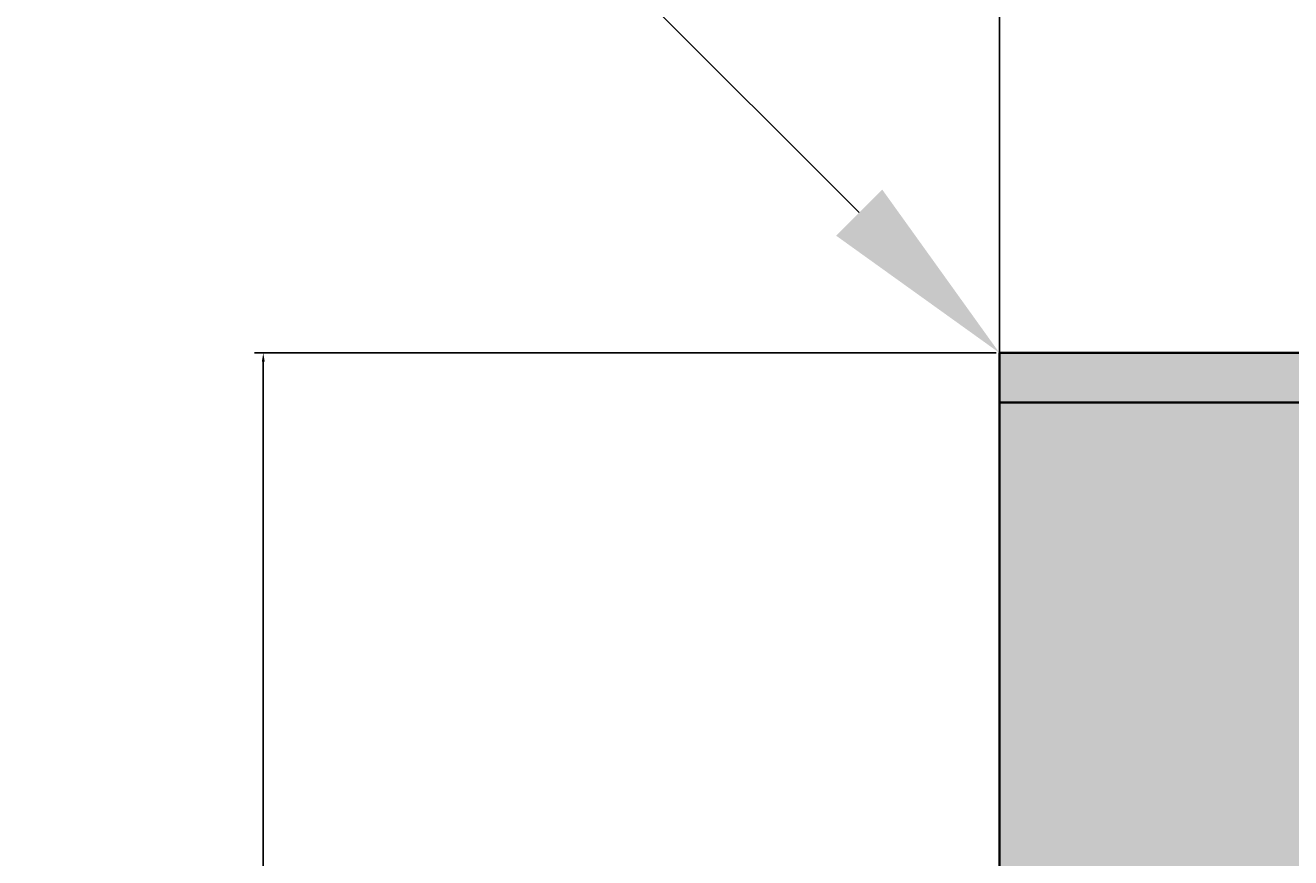
# Model space of a CAD drawing. Units: millimetres. Extents: x -11 to 280, y -4 to 208.
# Tile 50 of 55: x 186 to 211, y 156 to 173. Entities that reach past the tile are written whole.
import ezdxf
from ezdxf import colors
from ezdxf.entities.mleader import LeaderData, LeaderLine
from ezdxf.math import Vec2, Vec3

# ---------------------------------------------------------------- set-up
doc = ezdxf.new("R2010")
doc.units = ezdxf.units.MM
for name, color, linetype, lineweight in [('M-ANNO-TEXT', 7, 'Continuous', 18), ('M-DIMS', 2, 'Continuous', 18), ('M-HYDR-EQPM', 7, 'Continuous', 35), ('M-HYDR-EQPM-PATT', 252, 'Continuous', 13)]:
    doc.layers.add(name, color=color, linetype=linetype, lineweight=lineweight)
doc.styles.get("Standard").update_dxf_attribs({"font": 'arial.ttf'})
doc.dimstyles.get("Standard").update_dxf_attribs({"dimtxt": 0.18, "dimasz": 0.18, "dimexe": 0.18, "dimexo": 0.0625, "dimgap": 0.09, "dimtad": 0, "dimtih": 1, "dimtoh": 1, "dimdec": 4, "dimzin": 0, "dimdsep": 46, "dimtxsty": 'Standard', "dimcen": 0.09, "dimadec": 0, "dimazin": 0, "dimtfac": 1, "dimtdec": 4, "dimtofl": 0, "dimtmove": 0, "dimatfit": 3, "dimfxl": 1, "dimtolj": 1, "dimtzin": 0, "dimarcsym": 0})

# ---------------------------------------------------------------- blocks, each defined once
blk = doc.blocks.new('*D5')
at = {"layer": 'Defpoints', "color": 0, "transparency": 16777216}
for p in [(24.759, 192.645), (-10.087, 11.435), (261.686, 11.435)]:
    blk.add_point(p, dxfattribs=at)
at = {"layer": 'M-DIMS', "color": 0, "lineweight": -2, "transparency": 16777216}
for p, q in [((24.696, 192.645), (-10.267, 192.645)), ((-10.087, 192.465), (-10.087, 102.222)), ((-10.087, 11.615), (-10.087, 101.858)), ((261.624, 11.435), (-10.267, 11.435))]:
    blk.add_line(p, q, dxfattribs=at)
at = {"layer": 'M-DIMS', "color": 0, "transparency": 16777216}
for points in [[(-10.117, 192.465), (-10.057, 192.465), (-10.087, 192.645)], [(-10.117, 11.615), (-10.057, 11.615), (-10.087, 11.435)]]:
    blk.add_solid(points, dxfattribs=at)
at = {"layer": 'M-DIMS', "color": 0, "transparency": 16777216, "insert": (-10.087, 102.04), "char_height": 0.18, "attachment_point": 5}
blk.add_mtext('\\A1;181.2', dxfattribs=at)
blk = doc.blocks.new('*D6')
at = {"layer": 'Defpoints', "color": 0, "transparency": 16777216}
for p in [(236.935, 207.495), (66.388, 179.241), (236.935, 165.103)]:
    blk.add_point(p, dxfattribs=at)
at = {"layer": 'M-DIMS', "color": 0, "lineweight": -2, "transparency": 16777216}
for p, q in [((66.388, 179.304), (66.388, 207.675)), ((236.935, 165.166), (236.935, 207.675)), ((66.568, 207.495), (151.206, 207.495)), ((236.755, 207.495), (152.117, 207.495))]:
    blk.add_line(p, q, dxfattribs=at)
at = {"layer": 'M-DIMS', "color": 0, "transparency": 16777216}
for points in [[(66.568, 207.525), (66.568, 207.465), (66.388, 207.495)], [(236.755, 207.525), (236.755, 207.465), (236.935, 207.495)]]:
    blk.add_solid(points, dxfattribs=at)
at = {"layer": 'M-DIMS', "color": 0, "transparency": 16777216, "insert": (151.661, 207.495), "char_height": 0.18, "attachment_point": 5}
blk.add_mtext('\\A1;170.55', dxfattribs=at)
blk = doc.blocks.new('*D20')
at = {"layer": 'Defpoints', "color": 0, "transparency": 16777216}
for p in [(231.68, 207.495), (151.022, 43.599), (231.68, 43.599)]:
    blk.add_point(p, dxfattribs=at)
at = {"layer": 'M-DIMS', "color": 0, "lineweight": -2, "transparency": 16777216}
for p, q in [((151.022, 43.662), (151.022, 207.675)), ((231.68, 43.662), (231.68, 207.675)), ((151.202, 207.495), (190.957, 207.495)), ((231.5, 207.495), (191.745, 207.495))]:
    blk.add_line(p, q, dxfattribs=at)
at = {"layer": 'M-DIMS', "color": 0, "transparency": 16777216}
for points in [[(151.202, 207.525), (151.202, 207.465), (151.022, 207.495)], [(231.5, 207.525), (231.5, 207.465), (231.68, 207.495)]]:
    blk.add_solid(points, dxfattribs=at)
at = {"layer": 'M-DIMS', "color": 0, "transparency": 16777216, "insert": (191.351, 207.495), "char_height": 0.18, "attachment_point": 5}
blk.add_mtext('\\A1;80.66', dxfattribs=at)
blk = doc.blocks.new('*D25')
at = {"layer": 'Defpoints', "color": 0, "transparency": 16777216}
for p in [(236.935, 179.953), (205.531, 165.103), (236.935, 165.103)]:
    blk.add_point(p, dxfattribs=at)
at = {"layer": 'M-DIMS', "color": 0, "lineweight": -2, "transparency": 16777216}
for p, q in [((205.531, 165.166), (205.531, 180.133)), ((236.935, 165.166), (236.935, 180.133)), ((205.711, 179.953), (220.77, 179.953)), ((236.755, 179.953), (221.697, 179.953))]:
    blk.add_line(p, q, dxfattribs=at)
at = {"layer": 'M-DIMS', "color": 0, "transparency": 16777216}
for points in [[(205.711, 179.983), (205.711, 179.923), (205.531, 179.953)], [(236.755, 179.983), (236.755, 179.923), (236.935, 179.953)]]:
    blk.add_solid(points, dxfattribs=at)
at = {"layer": 'M-DIMS', "color": 0, "transparency": 16777216, "insert": (221.233, 179.953), "char_height": 0.18, "attachment_point": 5}
blk.add_mtext('\\A1;31.404', dxfattribs=at)
blk = doc.blocks.new('*D26')
at = {"layer": 'Defpoints', "color": 0, "transparency": 16777216}
for p in [(190.681, 166.103), (205.531, 166.103), (205.531, 144.661)]:
    blk.add_point(p, dxfattribs=at)
at = {"layer": 'M-DIMS', "color": 0, "lineweight": -2, "transparency": 16777216}
for p, q in [((205.469, 166.103), (190.501, 166.103)), ((190.681, 165.923), (190.681, 155.562)), ((190.681, 144.841), (190.681, 155.202)), ((205.469, 144.661), (190.501, 144.661))]:
    blk.add_line(p, q, dxfattribs=at)
at = {"layer": 'M-DIMS', "color": 0, "transparency": 16777216}
for points in [[(190.651, 165.923), (190.711, 165.923), (190.681, 166.103)], [(190.651, 144.841), (190.711, 144.841), (190.681, 144.661)]]:
    blk.add_solid(points, dxfattribs=at)
at = {"layer": 'M-DIMS', "color": 0, "transparency": 16777216, "insert": (190.681, 155.382), "char_height": 0.18, "attachment_point": 5}
blk.add_mtext('\\A1;21.442', dxfattribs=at)

msp = doc.modelspace()

# ---------------------------------------------------------------- hatches: boundary and pattern name
at = {"layer": 'M-HYDR-EQPM-PATT'}
h = msp.add_hatch(color=256, dxfattribs=at)
h.set_gradient(color1=(248, 153, 30), color2=(248, 153, 30), tint=1)
h.paths.add_polyline_path([(236.9353, 165.103), (205.5315, 165.103), (205.5315, 144.6609), (236.9353, 144.6609)])
h.paths.add_polyline_path([(244.8074, 166.103), (205.5315, 166.103), (205.5315, 165.103), (236.9353, 165.103), (245.4299, 165.103)])
h.paths.add_polyline_path([(248.3313, 165.603, -0.4142136), (248.8313, 166.103), (245.9853, 166.103), (246.6078, 165.103), (248.8313, 165.103, -0.4142136)])
h.paths.add_polyline_path([(249.3313, 165.603, 1), (248.3313, 165.603, 0.4142136), (248.8313, 165.103, 0.4142136)])

# ---------------------------------------------------------------- linework, layer by layer
at = {"layer": 'M-HYDR-EQPM'}
for p, q in [((205.5315, 166.103), (205.5315, 165.103)), ((244.8074, 166.103), (205.5315, 166.103))]:
    msp.add_line(p, q, dxfattribs=at)
msp.add_lwpolyline([(205.5315, 165.103), (236.9353, 165.103), (236.9353, 144.6609), (205.5315, 144.6609)], close=True, dxfattribs=at)

# ---------------------------------------------------------------- dimensions: what is measured, and where the dimension line sits
at = {"layer": 'M-DIMS'}
for base, p1, p2, override, picture, middle in [((236.9353, 207.495), (66.3875, 179.2412), (236.9353, 165.103), {"dimdec": 2, "dimlfac": 1, "dimrnd": 0, "dimzin": 0, "dimdsep": 46, "dimlunit": 2}, '*D6', (151.6614, 207.495)), ((231.6803, 207.495), (151.0217, 43.5991), (231.6803, 43.5991), {"dimdec": 2, "dimlfac": 1, "dimrnd": 0, "dimzin": 0, "dimdsep": 46, "dimlunit": 2}, '*D20', (191.351, 207.495)), ((236.9353, 179.953), (205.5315, 165.103), (236.9353, 165.103), {"dimdec": 3, "dimlfac": 1, "dimrnd": 0, "dimzin": 0, "dimdsep": 46, "dimlunit": 2}, '*D25', (221.2334, 179.953))]:
    dim = msp.add_linear_dim(base=base, p1=p1, p2=p2, dimstyle='Standard', override=override, dxfattribs=at)
    dim.commit()
    dim.dimension.update_dxf_attribs({"geometry": picture, "text_midpoint": middle})
for base, p1, p2, override, picture, middle in [((-10.0865, 11.4346), (24.7588, 192.645), (261.6863, 11.4346), {"dimdec": 1, "dimlfac": 1, "dimrnd": 0, "dimzin": 0, "dimdsep": 46, "dimlunit": 2}, '*D5', (-10.0865, 102.0398)), ((190.6815, 166.103), (205.5315, 144.6609), (205.5315, 166.103), {"dimdec": 3, "dimlfac": 1, "dimrnd": 0, "dimzin": 0, "dimdsep": 46, "dimlunit": 2}, '*D26', (190.6815, 155.382))]:
    dim = msp.add_linear_dim(base=base, p1=p1, p2=p2, angle=90, dimstyle='Standard', override=override, dxfattribs=at)
    dim.commit()
    dim.dimension.update_dxf_attribs({"geometry": picture, "text_midpoint": middle})

# ---------------------------------------------------------------- leaders
at = {"layer": 'M-ANNO-TEXT'}
ml = msp.add_multileader_mtext('Standard', dxfattribs=at)
ml.set_content('HAND PUMP', color=256)
ml.set_leader_properties()
ml.build(insert=Vec2(0, 0))
ctx = ml.context
ctx.base_point, ctx.plane_origin = Vec3(152.0312, 174.7629), Vec3(205.5315, 166.103)
ctx.text_align_type = 2
notes = []
notes.append((ctx, [(0, (1, 1, 0), (196.8716, 174.7629), (-1, 0), 8, [(0, [(205.5315, 166.103)], 0, [])])]))
ctx.mtext.insert, ctx.mtext.alignment, ctx.mtext.flow_direction = Vec3(186.8716, 176.7971), 3, 5
for ctx, leaders in notes:
    for number, flags, end, landing, length, lines in leaders:
        leader = LeaderData()
        leader.index, (leader.has_last_leader_line, leader.has_dogleg_vector, leader.attachment_direction) = number, flags
        leader.last_leader_point, leader.dogleg_vector, leader.dogleg_length = Vec3(end), Vec3(landing), length
        for number, points, colour, breaks in lines:
            line = LeaderLine()
            line.index, line.vertices, line.color, line.breaks = number, Vec3.list(points), colors.encode_raw_color(colour), breaks
            leader.lines.append(line)
        ctx.leaders.append(leader)

doc.saveas('drawing.dxf')
